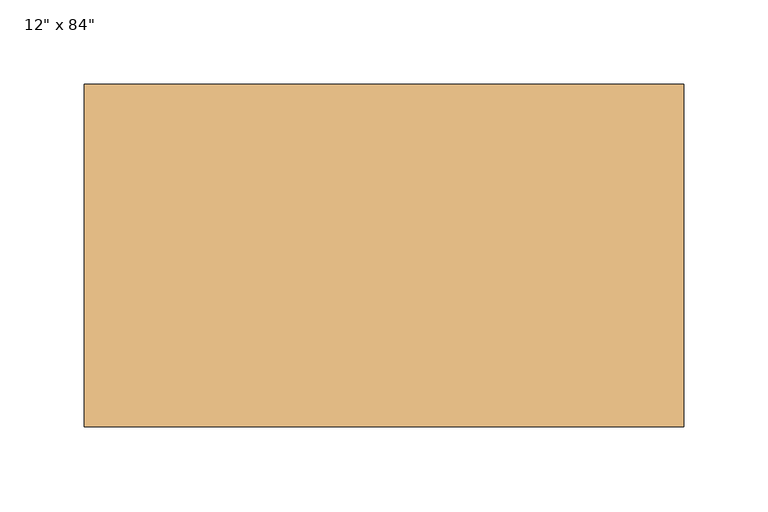
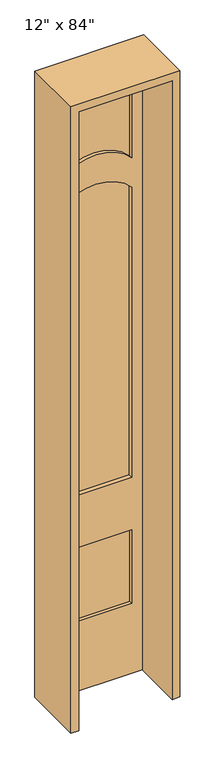
"""IFC4 building model written with IfcOpenShell, lengths in millimetres: door geometry."""

from ifc_helpers import new_model, si_unit, point, frame, frame_2d, origin, place, context, project, spatial, polyline, circle_curve, trimmed, segment, composite_curve, outline, extrude, source, transform, mapped, element, save


def door_c3736dc5(model_context):
    return source(origin(), model_context, "Body", "SweptSolid", [
        extrude(outline(polyline([(117.475, 75.1416667), (-117.475, 75.1416667), (-117.475, 86.7833333), (117.475, 86.7833333), (117.475, 75.1416667)])), frame((0.0, 0.0, 241.3), z_axis=(0.0, 0.0, 1.0), x_axis=(1.0, 0.0, 0.0)), (0.0, 0.0, 1.0), 254.0),
        extrude(outline(composite_curve([segment(polyline([(1778.0, 117.475), (2012.95, 117.475), (2012.95, -117.475), (1778.0, -117.475)]), True, "CONTINUOUS"), segment(trimmed(circle_curve(frame_2d((1667.5695312, 0.0)), 161.2304687), [point((1778.0, -117.475))], [point((1778.0, 117.475))], True, "CARTESIAN"), True, "CONTINUOUS")], self_intersect=False)), frame((0.0, 75.1416667, 0.0), z_axis=(0.0, 1.0, 0.0), x_axis=(0.0, 0.0, 1.0)), (0.0, 0.0, 1.0), 11.6416667),
        extrude(outline(polyline([(2133.6, -152.4), (0.0, -152.4), (0.0, 152.4), (2133.6, 152.4), (2133.6, -152.4)]), holes=[composite_curve([segment(polyline([(676.275, -117.475), (1676.4, -117.475)]), True, "CONTINUOUS"), segment(trimmed(circle_curve(frame_2d((1565.9695312, 0.0)), 161.2304688), [point((1676.4, -117.475))], [point((1676.4, 117.475))], True, "CARTESIAN"), True, "CONTINUOUS"), segment(polyline([(1676.4, 117.475), (676.275, 117.475), (676.275, -117.475)]), True, "CONTINUOUS")], self_intersect=False), polyline([(495.3, -117.475), (495.3, 117.475), (241.3, 117.475), (241.3, -117.475), (495.3, -117.475)]), composite_curve([segment(polyline([(2012.95, -117.475), (2012.95, 117.475), (1778.0, 117.475)]), True, "CONTINUOUS"), segment(trimmed(circle_curve(frame_2d((1667.5695312, 0.0)), 161.2304687), [point((1778.0, 117.475))], [point((1778.0, -117.475))], False, "CARTESIAN"), True, "CONTINUOUS"), segment(polyline([(1778.0, -117.475), (2012.95, -117.475)]), True, "CONTINUOUS")], self_intersect=False)]), frame((0.0, 63.5, 0.0), z_axis=(0.0, 1.0, 0.0), x_axis=(0.0, 0.0, 1.0)), (0.0, 0.0, 1.0), 34.925),
        extrude(outline(polyline([(0.0, 152.4), (0.0, 177.8), (2159.0, 177.8), (2159.0, -177.8), (0.0, -177.8), (0.0, -152.4), (2133.6, -152.4), (2133.6, 152.4), (0.0, 152.4)])), frame((0.0, -104.775, 0.0), z_axis=(0.0, 1.0, 0.0), x_axis=(0.0, 0.0, 1.0)), (0.0, 0.0, 1.0), 203.2),
        extrude(outline(composite_curve([segment(polyline([(676.275, -117.475), (676.275, 117.475), (1676.4, 117.475)]), True, "CONTINUOUS"), segment(trimmed(circle_curve(frame_2d((1565.9695312, 0.0)), 161.2304688), [point((1676.4, 117.475))], [point((1676.4, -117.475))], False, "CARTESIAN"), True, "CONTINUOUS"), segment(polyline([(1676.4, -117.475), (676.275, -117.475)]), True, "CONTINUOUS")], self_intersect=False)), frame((0.0, 77.47, 0.0), z_axis=(0.0, 1.0, 0.0), x_axis=(0.0, 0.0, 1.0)), (0.0, 0.0, 1.0), 6.985),
    ])


if __name__ == "__main__":
    model = new_model("IFC4")
    model_context = context("Model", 3, world=origin())
    ifc_project = project(units=[si_unit("LENGTHUNIT", "METRE", prefix="MILLI")], contexts=[model_context])
    site = spatial("IfcSite", under=ifc_project)
    building = spatial("IfcBuilding", under=site)
    placement = place(None, origin())
    door_shape = door_c3736dc5(model_context)
    element("IfcDoor", 1, ObjectType="12\" x 84\"", at=placement, inside=building, context=model_context, shape_type="MappedRepresentation", body=[
        mapped(door_shape, transform((0.0, 0.0, 0.0), x_axis=(1.0, 0.0, 0.0), y_axis=(0.0, 1.0, 0.0), z_axis=(0.0, 0.0, 1.0))),
    ])
    save(model, "model.ifc")

# Revit data of these elements
# Type "12\" x 84\""
#   Type Mark = "9"
#   Assembly Code = "B2030100"
#   Analytic Construction = "French door, wood frame with single glass"
#   Radius = 0' - 6 89/256"
#   Lock Rail = 0' - 7 1/8"
#   Thickness = 0' - 1 3/8"
#   Thermal Resistance (R) = 1.0696 (h·ft²·°F)/BTU
#   Stiles = 0' - 1 3/8"
#   Rough Width = 1' - 2"
#   Rough Height = 7' - 1"
#   Height = 7' - 0"
#   Width = 1' - 0"
#   Heat Transfer Coefficient (U) = 0.9350 BTU/(h·ft²·°F)
#   Door Offset [instance default] = 0' - 0"
#   Bottom Rail = 0' - 9 1/2"
#   Function = 1
#   Trim Material = Cherry
#   Panel Material = Cherry
#   Glazing = Glass
#   Frame Material = Cherry
#   Visual Light Transmittance = 0
#   Solar Heat Gain Coefficient = 0
#   Wall Closure = (empty or 0)
#   Construction Type = (empty or 0)
# Element 1 (IfcDoor, "12\" x 84\"")
#   Materials on its faces: "Cherry", "Glass"
# Materials
#   "Cherry": class "Wood", colour RGB 226 177 128, transparency 0, Description = "Prunus Serotina", Cost = 0
#   "Glass": class "Glass", colour RGB 0 128 192, transparency 0.75, Description = "Soda Lime Glass", Cost = 0
